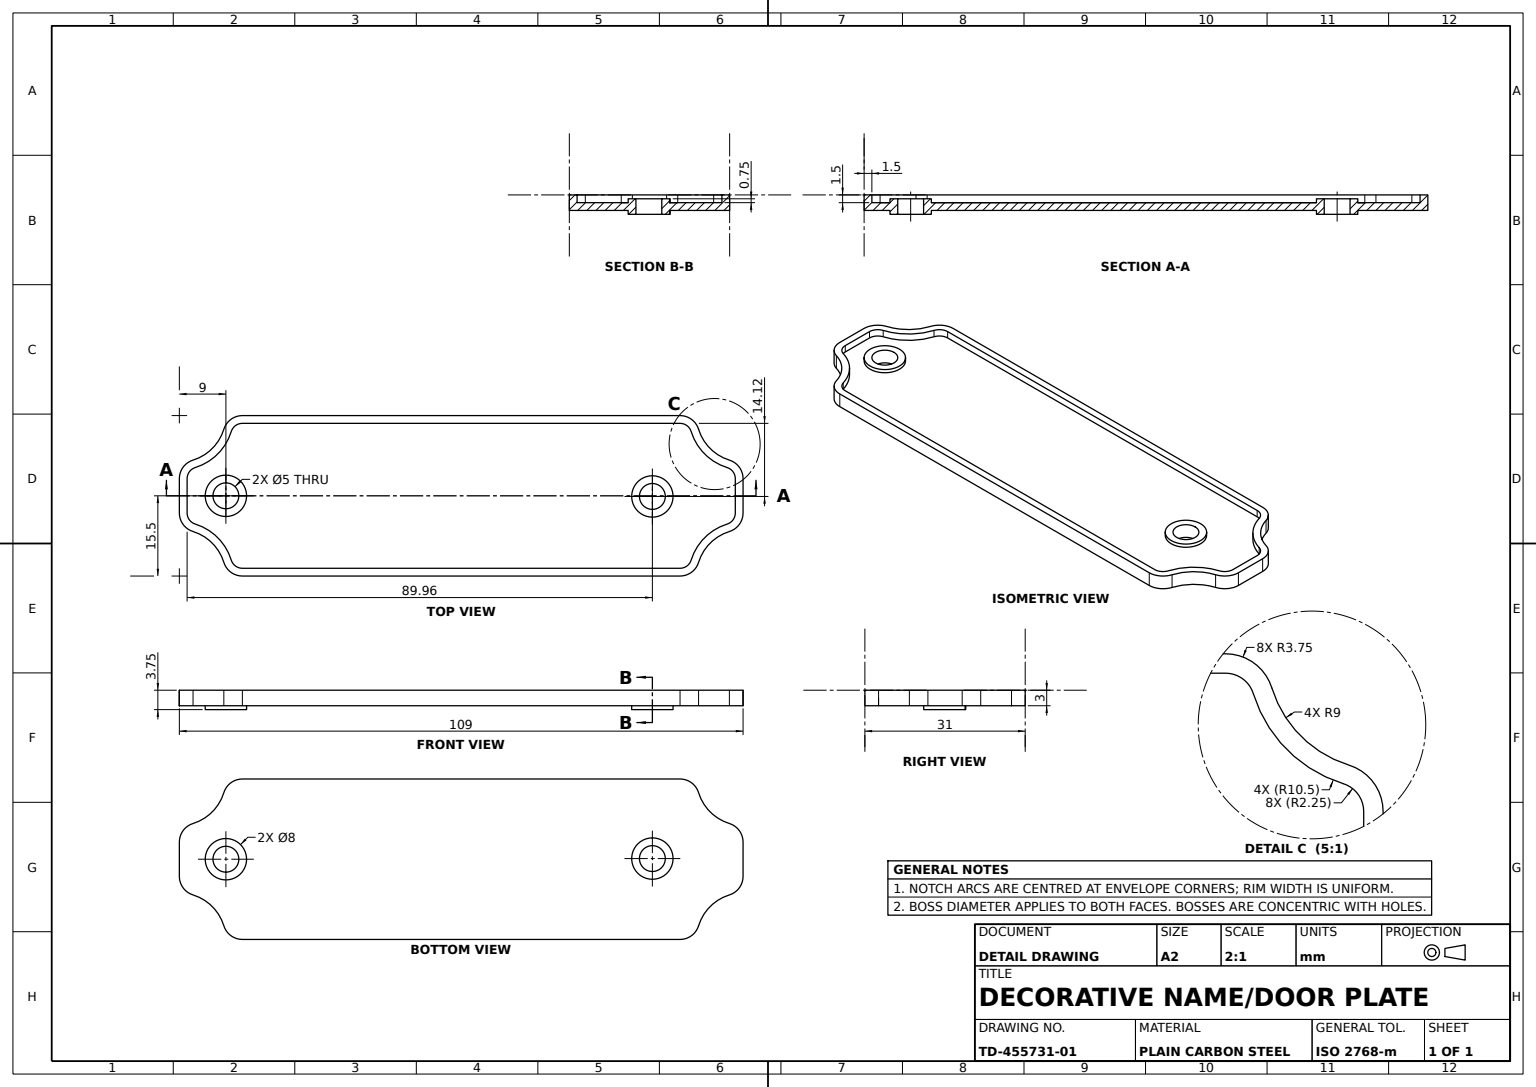
from build123d import *

# Parameters (mm, degrees)
BASE_PLATE_DEPTH                = 1.5
TOP_RECESS_1_5MM_DEPTH          = 1.5
MOUNTING_HOLE_BOSSES_DEPTH      = 0.75
MOUNTING_HOLE_BOSSES_DEPTH_BACK = 2.25
HOLE_BOSS_SKETCH_R              = 4
HOLE_BOSS_SKETCH_R_2            = 2.5
MOUNTING_HOLE_SKETCH_R          = 2.5
MOUNTING_HOLES_2X_DEPTH         = 30.75


with BuildPart() as part:
    # Plate Outline Sketch → Base Plate (new, symmetric)
    with BuildSketch(Plane(origin=(0, 0, 0), x_dir=(1, 0, 0), z_dir=(0, 1, 0))):
        with BuildLine():
            Line((-42.313942393, 15.5), (42.313942393, 15.5))
            ThreePointArc((42.313942393, 15.5), (44.541774365, 14.76649875), (45.898076983, 12.852941176))
            ThreePointArc((45.898076983, 12.852941176), (48.136038969, 9.136038969), (51.852941176, 6.898076983))
            ThreePointArc((51.852941176, 6.898076983), (53.76649875, 5.541774365), (54.5, 3.313942393))
            Line((54.5, 3.313942393), (54.5, -3.313942393))
            ThreePointArc((54.5, -3.313942393), (53.76649875, -5.541774365), (51.852941176, -6.898076983))
            ThreePointArc((51.852941176, -6.898076983), (48.136038969, -9.136038969), (45.898076983, -12.852941176))
            ThreePointArc((45.898076983, -12.852941176), (44.541774365, -14.76649875), (42.313942393, -15.5))
            Line((42.313942393, -15.5), (-42.313942393, -15.5))
            ThreePointArc((-42.313942393, -15.5), (-44.541774365, -14.76649875), (-45.898076983, -12.852941176))
            ThreePointArc((-45.898076983, -12.852941176), (-48.136038969, -9.136038969), (-51.852941176, -6.898076983))
            ThreePointArc((-51.852941176, -6.898076983), (-53.76649875, -5.541774365), (-54.5, -3.313942393))
            Line((-54.5, -3.313942393), (-54.5, 3.313942393))
            ThreePointArc((-54.5, 3.313942393), (-53.76649875, 5.541774365), (-51.852941176, 6.898076983))
            ThreePointArc((-51.852941176, 6.898076983), (-48.136038969, 9.136038969), (-45.898076983, 12.852941176))
            ThreePointArc((-45.898076983, 12.852941176), (-44.541774365, 14.76649875), (-42.313942393, 15.5))
        make_face()
    extrude(amount=BASE_PLATE_DEPTH, both=True)

    # Recess Outline Sketch → Top Recess 1.5mm (cut)
    with BuildSketch(Plane(origin=(0, 1.5, 0), x_dir=(1, 0, 0), z_dir=(0, 1, 0))):
        with BuildLine():
            Line((42.313942393, 14), (-42.313942393, 14))
            ThreePointArc((-42.313942393, 14), (-43.650641576, 13.55989925), (-44.464423147, 12.411764706))
            ThreePointArc((-44.464423147, 12.411764706), (-47.075378798, 8.075378798), (-51.411764706, 5.464423147))
            ThreePointArc((-51.411764706, 5.464423147), (-52.55989925, 4.650641576), (-53, 3.313942393))
            Line((-53, 3.313942393), (-53, -3.313942393))
            ThreePointArc((-53, -3.313942393), (-52.55989925, -4.650641576), (-51.411764706, -5.464423147))
            ThreePointArc((-51.411764706, -5.464423147), (-47.075378798, -8.075378798), (-44.464423147, -12.411764706))
            ThreePointArc((-44.464423147, -12.411764706), (-43.650641576, -13.55989925), (-42.313942393, -14))
            Line((-42.313942393, -14), (42.313942393, -14))
            ThreePointArc((42.313942393, -14), (43.650641576, -13.55989925), (44.464423147, -12.411764706))
            ThreePointArc((44.464423147, -12.411764706), (47.075378798, -8.075378798), (51.411764706, -5.464423147))
            ThreePointArc((51.411764706, -5.464423147), (52.55989925, -4.650641576), (53, -3.313942393))
            Line((53, -3.313942393), (53, 3.313942393))
            ThreePointArc((53, 3.313942393), (52.55989925, 4.650641576), (51.411764706, 5.464423147))
            ThreePointArc((51.411764706, 5.464423147), (47.075378798, 8.075378798), (44.464423147, 12.411764706))
            ThreePointArc((44.464423147, 12.411764706), (43.650641576, 13.55989925), (42.313942393, 14))
        make_face()
    extrude(amount=-TOP_RECESS_1_5MM_DEPTH, mode=Mode.SUBTRACT)

    # Hole Boss Sketch → Mounting Hole Bosses (add, two sides: drawn at the far end of the back side and taken through both)
    # profile 1 of 2: a face of its own
    with BuildSketch(Plane(origin=(0, 0, 0), x_dir=(1, 0, 0), z_dir=(0, 1, 0)).offset(-MOUNTING_HOLE_BOSSES_DEPTH_BACK)):
        with Locations(Location((-45.5, 0, 0), (0, 0, 270))):
            Circle(HOLE_BOSS_SKETCH_R)
        with Locations(Location((-45.5, 0, 0), (0, 0, 270))):
            Circle(HOLE_BOSS_SKETCH_R_2, mode=Mode.SUBTRACT)
    # profile 2 of 2: a face of its own
    with BuildSketch(Plane(origin=(0, 0, 0), x_dir=(1, 0, 0), z_dir=(0, 1, 0)).offset(-MOUNTING_HOLE_BOSSES_DEPTH_BACK)):
        with Locations(Location((36.963444552, -0.123211482, 0), (0, 0, 270))):
            Circle(HOLE_BOSS_SKETCH_R)
        with Locations(Location((36.963444552, -0.123211482, 0), (0, 0, 270))):
            Circle(HOLE_BOSS_SKETCH_R_2, mode=Mode.SUBTRACT)
    extrude(amount=MOUNTING_HOLE_BOSSES_DEPTH + MOUNTING_HOLE_BOSSES_DEPTH_BACK)

    # Mounting Hole Sketch → Mounting Holes 2x (cut)
    with BuildSketch(Plane(origin=(0, 0, 0), x_dir=(1, 0, 0), z_dir=(0, 1, 0))):
        with Locations(Location((36.963444552, -0.123211482, 0), (0, 0, 270))):
            Circle(MOUNTING_HOLE_SKETCH_R)
        with Locations(Location((-45.5, 0, 0), (0, 0, 270))):
            Circle(MOUNTING_HOLE_SKETCH_R)
    extrude(amount=-MOUNTING_HOLES_2X_DEPTH, mode=Mode.SUBTRACT)


solid = part.part
